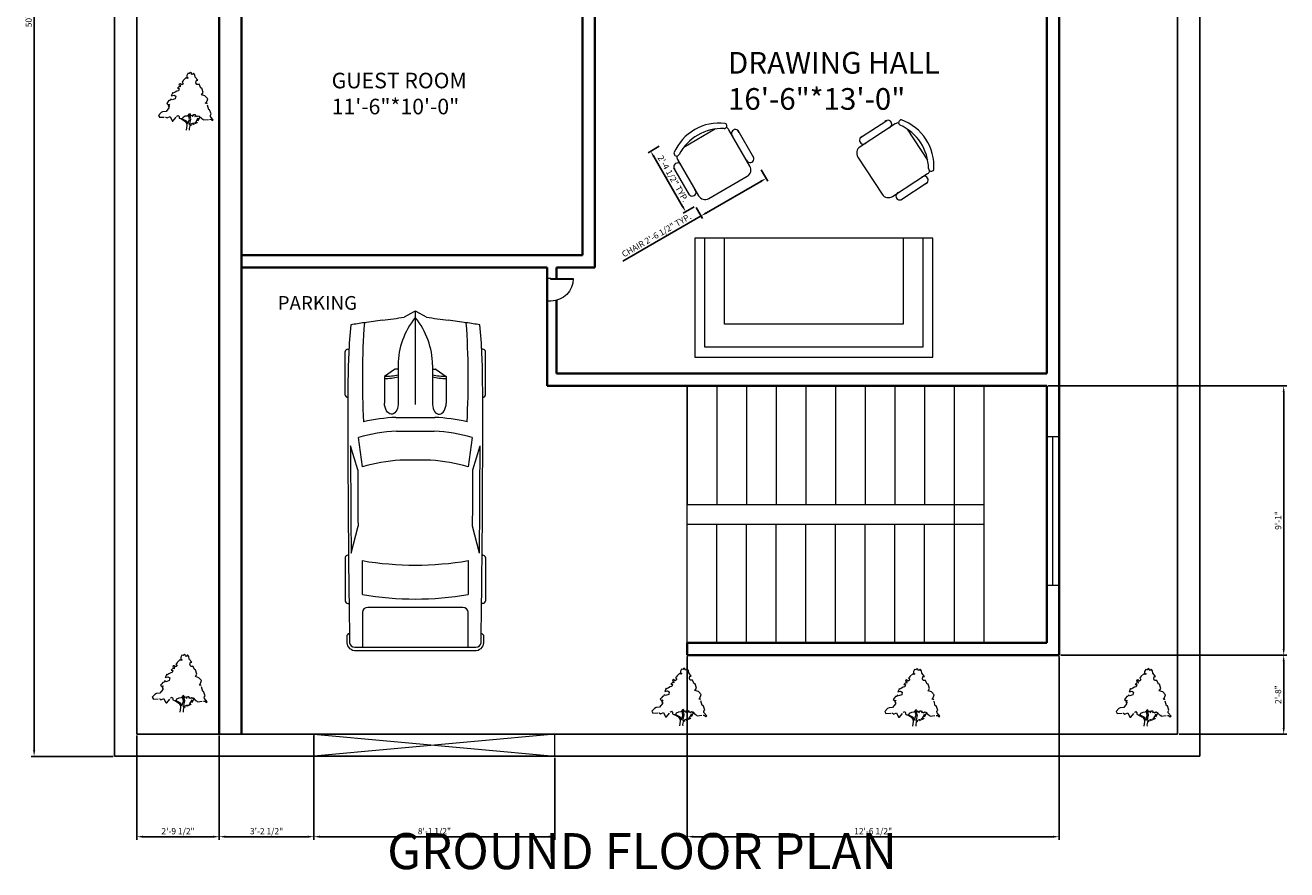
# Model space of a CAD drawing. Units: inches. Extents: x 2432 to 3786, y 1221 to 1905.
# Tile 1 of 4: x 2434 to 2945, y 1221 to 1563. Entities that reach past the tile are written whole.
import ezdxf

# ---------------------------------------------------------------- set-up
doc = ezdxf.new("R2010")
doc.units = ezdxf.units.IN
doc.linetypes.add('ACAD_ISO02W100', pattern=[15, 12, -3])
for name, color, linetype, lineweight, true_color in [('A-ANNO-DIMS', 32, 'Continuous', 18, 0xcd6928), ('A-ANNO-TITL', 40, 'Continuous', 25, 0xf8d731), ('A-AREA-IDEN', 244, 'Continuous', 18, 0x991b1e), ('A-FLOR-STRS', 116, 'Continuous', 18, 0x136734), ('A-FURN', 32, 'Continuous', 13, 0xcd6928), ('A-GLAZ', 116, 'Continuous', 18, 0x136734), ('A-WALL', 67, 'Continuous', 35, 0x727430), ('C-PROP', 67, 'Continuous', 25, 0x727430), ('L-SITE-GATE', 244, 'Continuous', 18, 0x991b1e)]:
    doc.layers.add(name, color=color, linetype=linetype, lineweight=lineweight, true_color=true_color)
for name, color, linetype, lineweight in [('A-DOOR', 4, 'Continuous', 18), ('C-PRKG-VEHC', 8, 'Continuous', 13), ('L-PLNT', 3, 'ACAD_ISO02W100', 13)]:
    doc.layers.add(name, color=color, linetype=linetype, lineweight=lineweight)
doc.styles.get("Standard").update_dxf_attribs({"font": 'arial.ttf'})
doc.dimstyles.new('ISO-25', dxfattribs={"dimtxt": 2.5, "dimasz": 2.5, "dimexe": 1.25, "dimexo": 0.625, "dimtad": 1, "dimdec": 3, "dimlunit": 4, "dimtxsty": 'Standard', "dimcen": 2.5, "dimadec": 0, "dimazin": 0, "dimtfac": 1, "dimtdec": 3, "dimtmove": 0, "dimatfit": 3, "dimfxl": 1, "dimarcsym": 0})

# ---------------------------------------------------------------- blocks, each defined once
blk = doc.blocks.new('*U2')
for p, q in [((21.1, 37.41), (21.1, 36.83)), ((46.55, 38.89), (22.35, 38.89)), ((47.8, 37.39), (47.8, 37.41)), ((87.99, 31.87), (74.76, 35.92)), ((134.31, 35.6), (119.29, 31.78)), ((135.45, 37.07), (135.45, 37.41)), ((136.7, 38.89), (160.9, 38.89)), ((162.15, 37.41), (162.15, 36.77)), ((70.03, 31.54), (86.41, 29.35)), ((138.42, 29.35), (157.25, 29.35)), ((186.47, 29.35), (167.01, 29.35)), ((186.47, -33.5), (186.47, 33.5)), ((188.4, -32.76), (188.4, 32.76)), ((164.52, 26.39), (164.52, -26.39)), ((32.27, 11.63), (36.13, 17.17)), ((36.13, 17.17), (50.94, 17.17)), ((29.77, 9.51), (51.68, 9.51)), ((32.12, 9.51), (32.12, 11.15)), ((58.92, -10.77), (58.92, 10.77)), ((66.55, -10.53), (66.55, 10.53)), ((82.74, 8.5), (82.74, -8.5)), ((186.47, -10.53), (186.47, 10.53)), ((3.27, 6.13), (0.1, 0.41)), ((0, 0), (51.68, 0)), ((0.1, -0.41), (3.27, -6.13)), ((29.77, -9.51), (51.68, -9.51)), ((32.12, -9.51), (32.12, -11.15)), ((32.27, -11.63), (36.13, -17.17)), ((36.13, -17.17), (50.94, -17.17)), ((86.41, -29.35), (70.03, -31.54)), ((87.99, -31.87), (74.76, -35.92)), ((134.31, -35.6), (119.29, -31.78)), ((157.25, -29.35), (138.42, -29.35)), ((167.01, -29.35), (186.47, -29.35)), ((21.1, -37.41), (21.1, -36.83)), ((46.55, -38.89), (22.35, -38.89)), ((47.8, -37.39), (47.8, -37.41)), ((135.45, -37.07), (135.45, -37.41)), ((136.7, -38.89), (160.9, -38.89)), ((162.15, -37.41), (162.15, -36.77))]:
    blk.add_line(p, q)
for centre, major_axis, ratio, start_param, end_param in [((266.03, -27.52), (0, 313.31), 0.842304, 1.367076, 1.39176), ((41.19, -490.86), (0, 528.23), 0.842304, 0.00281, 0.075598), ((22.35, 37.41), (0, -1.48), 0.842304, 3.141593, 4.712389), ((64.48, -10555.62), (0, 10593.03), 0.842304, -0.013397, 0.002797), ((46.55, 37.41), (0, 1.48), 0.842304, -1.570796, 0), ((64.48, -10555.62), (0, -10591.55), 0.842304, 3.133765, 3.140441), ((136.7, 37.41), (0, -1.48), 0.842304, 3.141593, 4.712389), ((160.9, 37.41), (0, 1.48), 0.842304, -1.570796, 0), ((180.63, 35.84), (0, 2.22), 0.842304, -0.013017, 1.249894), ((64.48, -10556.36), (0, 10595.31), 0.842304, -0.013397, -0.013017), ((183.98, 33.5), (0, -2.96), 0.842304, 1.570796, 3.128196), ((183.98, 32.76), (0, -5.25), 0.842304, 1.570796, 3.128196), ((259.18, -27.52), (0, -305.3), 0.842304, 4.528606, 4.561838), ((37.47, -593.96), (0, -623.33), 0.842304, 3.096046, 3.200911), ((134.4, 5.39), (0, -89.78), 0.842304, 4.449482, 4.652344), ((135.29, 5.39), (0, 81.77), 0.842304, 1.245306, 1.50788), ((149.6, 2.8), (0, -79.58), 0.842304, 4.372215, 4.640744), ((95.79, -3666.35), (0, -3698.24), 0.842304, 3.134049, 3.144098), ((17.08, 0), (0, 147.02), 0.842304, 4.511394, 4.913384), ((35.91, 0), (0, 147.02), 0.842304, 4.511394, 4.913384), ((167.01, 26.39), (0, 2.96), 0.842304, 0, 1.570796), ((-204.49, 52.4), (0, -250.96), 0.842304, 1.385369, 1.434372), ((13.04, 17.01), (0, 27.42), 0.842304, 4.435146, 4.718221), ((14.2, 17.01), (0, 27.42), 0.842304, 4.435146, 4.718221), ((50.79, 13.34), (6.34, -0.36), 0.603834, -1.395552, 1.581315), ((29.77, -46.66), (0, 56.17), 0.842304, 0, 0.590319), ((32.75, 11.15), (0, 0.74), 0.842304, 0.879714, 1.570796), ((0.62, 0), (0, -0.74), 0.842304, 4.131459, 5.293319), ((-204.49, -52.4), (0, 250.96), 0.842304, -1.434372, -1.385369), ((29.77, 46.66), (0, 56.17), 0.842304, 2.551274, 3.141593), ((32.75, -11.15), (0, -0.74), 0.842304, 4.712389, 5.403472), ((13.04, -17.01), (0, -27.42), 0.842304, 1.564964, 1.848039), ((14.2, -17.01), (0, -27.42), 0.842304, 1.564964, 1.848039), ((134.4, -5.39), (0, -89.78), 0.842304, -1.510751, -1.307889), ((135.29, -5.39), (0, -81.77), 0.842304, -1.50788, -1.245306), ((149.6, -2.8), (0, -79.58), 0.842304, -1.499151, -1.230623), ((259.18, 27.52), (0, 305.3), 0.842304, 1.721348, 1.754579), ((167.01, -26.39), (0, -2.96), 0.842304, 4.712389, 6.283185), ((266.03, 27.52), (0, 313.31), 0.842304, 1.749832, 1.774517), ((37.47, 593.96), (0, -623.33), 0.842304, -0.059319, 0.045547), ((95.79, 3666.35), (0, -3698.24), 0.842304, -0.002505, 0.007544), ((183.98, -33.5), (0, 2.96), 0.842304, 3.15499, 4.712389), ((183.98, -32.76), (0, -5.25), 0.842304, 0.013397, 1.570796), ((41.19, 490.86), (0, -528.23), 0.842304, -0.075598, -0.00281), ((22.35, -37.41), (0, 1.48), 0.842304, 1.570796, 3.141593), ((64.48, 10555.62), (0, 10593.03), 0.842304, 3.138796, 3.15499), ((46.55, -37.41), (0, -1.48), 0.842304, 0, 1.570796), ((64.48, 10555.62), (0, -10591.55), 0.842304, 0.001152, 0.007828), ((136.7, -37.41), (0, -1.48), 0.842304, -1.570796, 0), ((160.9, -37.41), (0, 1.48), 0.842304, 3.141593, 4.712389), ((180.63, -35.84), (0, -2.22), 0.842304, -1.249894, 0.013017), ((64.48, 10556.36), (0, 10595.31), 0.842304, 3.15461, 3.15499)]:
    blk.add_ellipse(centre, major_axis=major_axis, ratio=ratio, start_param=start_param, end_param=end_param)
at = {"extrusion": (0, 0, -1)}
blk.add_ellipse((50.79, -13.34), major_axis=(6.34, 0.36), ratio=0.603834, start_param=-1.395552, end_param=1.581315, dxfattribs=at)
blk = doc.blocks.new('*U4')
for points in [[(22.0124, 137.721), (18.5475, 141.5624), (15.5282, 138.2446), (13.8028, 139.3505), (13.3714, 142.1153), (11.2148, 143.2214), (8.1954, 140.4564), (4.7447, 141.0094), (2.1567, 136.0326), (2.1567, 131.6088), (5.6074, 129.9499), (3.0193, 128.2909), (0.4313, 130.5029), (-6.9015, 123.3141), (-6.9015, 121.6552), (-9.9208, 119.9963), (-9.0581, 118.3373), (-6.9015, 115.0195), (-10.7835, 112.2546), (-14.6656, 115.0195), (-16.8222, 114.4665), (-17.6849, 112.2546), (-14.6656, 111.7016), (-14.2342, 107.2778), (-17.6065, 107.8307), (-21.5669, 103.9599), (-17.2536, 103.4069), (-18.9789, 97.8771), (-22.8609, 97.3241), (-27.1743, 94.5593), (-32.3504, 91.7944), (-32.7817, 94.0063), (-36.6638, 85.7116), (-29.7624, 87.3705), (-25.449, 84.6056), (-26.743, 77.9699), (-34.507, 75.205), (-37.9578, 77.4169), (-39.2518, 74.099), (-42.2711, 73.5461), (-44.8592, 70.2282), (-47.8786, 66.3574), (-43.9965, 63.0395), (-41.4085, 64.6985), (-44.3346, 59.8898), (-42.2089, 60.1377), (-42.5159, 55.7849), (-49.6039, 46.4502), (-58.2307, 45.8972), (-62.1127, 43.6853), (-68.5828, 36.4966), (-65.9947, 32.0727), (-50.0352, 32.6257), (-47.0159, 30.4138), (-39.6831, 33.7317), (-34.507, 22.6721), (-32.3504, 22.6721), (-22.4296, 34.8376), (-19.4102, 36.4966), (-17.2536, 33.7317), (-17.2536, 29.8608), (-13.8028, 28.7549), (-9.0581, 28.7549), (-7.3328, 32.6257), (-1.7254, 35.3906), (3.8821, 35.9436), (6.4701, 38.1555), (6.9014, 38.7085), (8.1954, 41.4734), (9.9208, 40.3674), (11.2148, 35.9436), (14.2341, 37.6025), (15.0968, 36.4966), (15.9595, 33.7317), (18.9789, 38.7085), (21.9982, 38.7085), (23.2922, 36.4966), (21.9982, 34.2847), (25.4489, 35.3906), (26.743, 33.7317), (29.7623, 35.9436), (32.7817, 34.8376), (38.8204, 28.7549), (41.4084, 27.6489), (43.5651, 25.437), (61.6813, 27.0959), (65.132, 23.7781), (67.7201, 24.884), (60.8186, 33.7317), (60.3873, 37.0495), (62.544, 40.3674), (58.662, 50.874), (56.5053, 50.874), (52.1919, 66.3574), (47.8785, 66.9103), (50.4665, 69.1222), (53.9172, 77.9699), (47.0158, 85.1586), (38.3891, 87.9235), (42.2711, 94.0063)], [(42.2711, 94.0063), (38.8204, 104.5129), (36.6637, 104.5129), (32.3503, 113.9135), (29.7623, 113.3605), (26.743, 113.3605), (24.5862, 117.7844), (25.8802, 123.8671), (29.331, 123.8671), (22.8609, 131.6088), (21.9982, 137.6916)], [(-9.9208, 28.2019), (0, 23.2251), (3.4507, 19.9072), (4.7447, 15.4834), (8.6267, 27.0959), (6.4701, 37.6025)], [(34.5071, 33.1787), (27.1743, 18.2483), (9.0581, 10.5066), (7.7641, 3.8708), (8.1954, 0)], [(8.1954, 40.3674), (11.2148, 27.6489), (8.1954, 13.8245), (24.5862, 19.9072), (32.7817, 34.2847)], [(-12.9401, 28.7549), (-2.588, 22.1191), (0.8626, 17.6953), (1.7253, 11.6125), (0, 0)]]:
    blk.add_lwpolyline(points)
blk = doc.blocks.new('SOFA2')
for p, q in [((-36, 0), (-36, -36)), ((36, 0), (-36, 0)), ((36, -36), (36, 0)), ((-33, -36), (-33, -3)), ((-33, -3), (33, -3)), ((33, -3), (33, -36)), ((-27, -36), (-27, -10)), ((-27, -10), (27, -10)), ((27, -10), (27, -36)), ((-36, -36), (36, -36))]:
    blk.add_line(p, q)
blk = doc.blocks.new('CHAIR7')
for p, q in [((20, 12), (3, 12)), ((5.12, 15.04), (17.88, 15.04)), ((0, 9), (0, -9)), ((23, -7.44), (23, 7.44)), ((3, -12), (20, -12)), ((5.12, -15), (17.88, -15))]:
    blk.add_line(p, q)
for centre, radius, start, end in [((3, 9), 3, 90, 180), ((5.56, 13.54), 1.56, 73.7398, 286.2602), ((17.44, 13.54), 1.56, 253.7398, 106.2602), ((20, 9), 3, 62.4156, 90), ((22.34, 11.12), 1.1, 53.3099, 212.0274), ((4.82, 0), 19.64, 327.5758, 32.4242), ((7, 0), 20, 323.1301, 36.8699), ((3, -9), 3, 180, 270), ((5.56, -13.5), 1.56, 73.7398, 286.2602), ((17.44, -13.5), 1.56, 253.7398, 106.2602), ((20, -9), 3, 270, 297.5844), ((22.34, -11.12), 1.1, 147.9726, 306.6901)]:
    blk.add_arc(centre, radius, start, end)
blk = doc.blocks.new('*U10')
for p, q in [((0, 0), (0, -6)), ((-40, 0), (-40, -6))]:
    blk.add_line(p, q)
blk.add_lwpolyline([(0, 0), (0, 40), (-1.75, 40), (-1.75, 0)], close=True)
blk.add_arc((0, 0), 40, 90, 180)
blk = doc.blocks.new('*D19')
at = {"layer": 'A-ANNO-DIMS', "color": 0, "lineweight": -2, "transparency": 16777216}
for p, q in [((2732.23, 1504.76), (2734.82, 1500.27)), ((2732.03, 1500.1), (2710.02, 1487.39)), ((2705.89, 1489.55), (2708.48, 1485.06)), ((2707.86, 1486.14), (2676.14, 1467.83))]:
    blk.add_line(p, q, dxfattribs=at)
at = {"layer": 'A-ANNO-DIMS', "color": 0, "lineweight": 5, "transparency": 16777216}
for points in [[(2731.82, 1500.46), (2732.24, 1499.74), (2734.2, 1501.35)], [(2709.81, 1487.76), (2710.23, 1487.03), (2707.86, 1486.14)]]:
    blk.add_solid(points, dxfattribs=at)
at = {"layer": 'Defpoints', "color": 0, "lineweight": 5, "transparency": 16777216}
for p in [(2731.92, 1505.3), (2705.58, 1490.1), (2707.86, 1486.14)]:
    blk.add_point(p, dxfattribs=at)
at = {"layer": 'A-ANNO-DIMS', "color": 0, "transparency": 16777216, "insert": (2689.96, 1478.03), "char_height": 2.5, "attachment_point": 5, "rotation": 30}
blk.add_mtext('CHAIR 2\'-6 1/2" TYP.', dxfattribs=at)
blk = doc.blocks.new('*D20')
at = {"layer": 'A-ANNO-DIMS', "color": 0, "lineweight": -2, "transparency": 16777216}
for p, q in [((2690.87, 1514.32), (2686.38, 1511.73)), ((2700.38, 1489.98), (2688.71, 1510.19)), ((2705.04, 1489.78), (2700.54, 1487.19))]:
    blk.add_line(p, q, dxfattribs=at)
at = {"layer": 'A-ANNO-DIMS', "color": 0, "lineweight": 5, "transparency": 16777216}
for points in [[(2689.07, 1510.4), (2688.35, 1509.98), (2687.46, 1512.35)], [(2700.74, 1490.19), (2700.02, 1489.77), (2701.63, 1487.81)]]:
    blk.add_solid(points, dxfattribs=at)
at = {"layer": 'Defpoints', "color": 0, "lineweight": 5, "transparency": 16777216}
for p in [(2687.46, 1512.35), (2691.41, 1514.63), (2705.58, 1490.1)]:
    blk.add_point(p, dxfattribs=at)
at = {"layer": 'A-ANNO-DIMS', "color": 0, "transparency": 16777216, "insert": (2696.2, 1501.04), "char_height": 2.5, "attachment_point": 5, "rotation": 300}
blk.add_mtext('2\'-4 1/2" TYP.', dxfattribs=at)
blk = doc.blocks.new('*D36')
at = {"layer": 'A-ANNO-DIMS', "color": 0, "lineweight": -2, "transparency": 16777216}
for p, q in [((2469.77, 1867.25), (2436.59, 1867.25)), ((2437.84, 1269.75), (2437.84, 1864.75)), ((2469.77, 1267.25), (2436.59, 1267.25))]:
    blk.add_line(p, q, dxfattribs=at)
at = {"layer": 'A-ANNO-DIMS', "color": 0, "lineweight": 5, "transparency": 16777216}
for points in [[(2437.42, 1864.75), (2438.26, 1864.75), (2437.84, 1867.25)], [(2437.42, 1269.75), (2438.26, 1269.75), (2437.84, 1267.25)]]:
    blk.add_solid(points, dxfattribs=at)
at = {"layer": 'Defpoints', "color": 0, "lineweight": 5, "transparency": 16777216}
for p in [(2437.84, 1867.25), (2470.39, 1867.25), (2470.39, 1267.25)]:
    blk.add_point(p, dxfattribs=at)
at = {"layer": 'A-ANNO-DIMS', "color": 0, "transparency": 16777216, "insert": (2435.94, 1567.25), "char_height": 2.5, "attachment_point": 5, "rotation": 90}
blk.add_mtext('50\'-0"', dxfattribs=at)
blk = doc.blocks.new('*D37')
at = {"layer": 'A-ANNO-DIMS', "color": 0, "lineweight": -2, "transparency": 16777216}
for p, q in [((2479.39, 1275.63), (2479.39, 1233.45)), ((2512.8, 1275.63), (2512.8, 1233.45)), ((2481.89, 1234.7), (2510.3, 1234.7))]:
    blk.add_line(p, q, dxfattribs=at)
at = {"layer": 'A-ANNO-DIMS', "color": 0, "lineweight": 5, "transparency": 16777216}
for points in [[(2481.89, 1235.12), (2481.89, 1234.28), (2479.39, 1234.7)], [(2510.3, 1235.12), (2510.3, 1234.28), (2512.8, 1234.7)]]:
    blk.add_solid(points, dxfattribs=at)
at = {"layer": 'Defpoints', "color": 0, "lineweight": 5, "transparency": 16777216}
for p in [(2479.39, 1276.25), (2512.8, 1276.25), (2512.8, 1234.7)]:
    blk.add_point(p, dxfattribs=at)
at = {"layer": 'A-ANNO-DIMS', "color": 0, "transparency": 16777216, "insert": (2496.09, 1236.62), "char_height": 2.5, "attachment_point": 5}
blk.add_mtext('2\'-9 1/2"', dxfattribs=at)
blk = doc.blocks.new('*D38')
at = {"layer": 'A-ANNO-DIMS', "color": 0, "lineweight": -2, "transparency": 16777216}
for p, q in [((2848.42, 1417.25), (2944.97, 1417.25)), ((2943.72, 1310.75), (2943.72, 1414.75)), ((2853.45, 1308.25), (2944.97, 1308.25))]:
    blk.add_line(p, q, dxfattribs=at)
at = {"layer": 'A-ANNO-DIMS', "color": 0, "lineweight": 5, "transparency": 16777216}
for points in [[(2943.31, 1414.75), (2944.14, 1414.75), (2943.72, 1417.25)], [(2943.31, 1310.75), (2944.14, 1310.75), (2943.72, 1308.25)]]:
    blk.add_solid(points, dxfattribs=at)
at = {"layer": 'Defpoints', "color": 0, "lineweight": 5, "transparency": 16777216}
for p in [(2847.8, 1417.25), (2943.72, 1417.25), (2852.82, 1308.25)]:
    blk.add_point(p, dxfattribs=at)
at = {"layer": 'A-ANNO-DIMS', "color": 0, "transparency": 16777216, "insert": (2941.82, 1362.75), "char_height": 2.5, "attachment_point": 5, "rotation": 90}
blk.add_mtext('9\'-1"', dxfattribs=at)
blk = doc.blocks.new('*D39')
at = {"layer": 'A-ANNO-DIMS', "color": 0, "lineweight": -2, "transparency": 16777216}
for p, q in [((2853.45, 1308.25), (2944.97, 1308.25)), ((2943.72, 1305.75), (2943.72, 1278.75)), ((2901.42, 1276.25), (2944.97, 1276.25))]:
    blk.add_line(p, q, dxfattribs=at)
at = {"layer": 'A-ANNO-DIMS', "color": 0, "lineweight": 5, "transparency": 16777216}
for points in [[(2943.31, 1305.75), (2944.14, 1305.75), (2943.72, 1308.25)], [(2943.31, 1278.75), (2944.14, 1278.75), (2943.72, 1276.25)]]:
    blk.add_solid(points, dxfattribs=at)
at = {"layer": 'Defpoints', "color": 0, "lineweight": 5, "transparency": 16777216}
for p in [(2852.82, 1308.25), (2900.8, 1276.25), (2943.72, 1276.25)]:
    blk.add_point(p, dxfattribs=at)
at = {"layer": 'A-ANNO-DIMS', "color": 0, "transparency": 16777216, "insert": (2941.82, 1292.25), "char_height": 2.5, "attachment_point": 5, "rotation": 90}
blk.add_mtext('2\'-8"', dxfattribs=at)
blk = doc.blocks.new('*D40')
at = {"layer": 'A-ANNO-DIMS', "color": 0, "lineweight": -2, "transparency": 16777216}
for p, q in [((2702.21, 1307.62), (2702.21, 1233.45)), ((2852.82, 1307.63), (2852.82, 1233.45)), ((2704.71, 1234.7), (2850.32, 1234.7))]:
    blk.add_line(p, q, dxfattribs=at)
at = {"layer": 'A-ANNO-DIMS', "color": 0, "lineweight": 5, "transparency": 16777216}
for points in [[(2704.71, 1235.12), (2704.71, 1234.28), (2702.21, 1234.7)], [(2850.32, 1235.12), (2850.32, 1234.28), (2852.82, 1234.7)]]:
    blk.add_solid(points, dxfattribs=at)
at = {"layer": 'Defpoints', "color": 0, "lineweight": 5, "transparency": 16777216}
for p in [(2702.21, 1308.25), (2852.82, 1308.25), (2852.82, 1234.7)]:
    blk.add_point(p, dxfattribs=at)
at = {"layer": 'A-ANNO-DIMS', "color": 0, "transparency": 16777216, "insert": (2777.52, 1236.62), "char_height": 2.5, "attachment_point": 5}
blk.add_mtext('12\'-6 1/2"', dxfattribs=at)
blk = doc.blocks.new('*D41')
at = {"layer": 'A-ANNO-DIMS', "color": 0, "lineweight": -2, "transparency": 16777216}
for p, q in [((2551.09, 1266.63), (2551.09, 1233.45)), ((2648.7, 1266.63), (2648.7, 1233.45)), ((2553.59, 1234.7), (2646.2, 1234.7))]:
    blk.add_line(p, q, dxfattribs=at)
at = {"layer": 'A-ANNO-DIMS', "color": 0, "lineweight": 5, "transparency": 16777216}
for points in [[(2553.59, 1235.12), (2553.59, 1234.28), (2551.09, 1234.7)], [(2646.2, 1235.12), (2646.2, 1234.28), (2648.7, 1234.7)]]:
    blk.add_solid(points, dxfattribs=at)
at = {"layer": 'Defpoints', "color": 0, "lineweight": 5, "transparency": 16777216}
for p in [(2551.09, 1267.25), (2648.7, 1267.25), (2648.7, 1234.7)]:
    blk.add_point(p, dxfattribs=at)
at = {"layer": 'A-ANNO-DIMS', "color": 0, "transparency": 16777216, "insert": (2599.9, 1236.62), "char_height": 2.5, "attachment_point": 5}
blk.add_mtext('8\'-1 1/2"', dxfattribs=at)
blk = doc.blocks.new('*D42')
at = {"layer": 'A-ANNO-DIMS', "color": 0, "lineweight": -2, "transparency": 16777216}
for p, q in [((2512.8, 1275.63), (2512.8, 1233.45)), ((2551.09, 1275.63), (2551.09, 1233.45)), ((2515.3, 1234.7), (2548.59, 1234.7))]:
    blk.add_line(p, q, dxfattribs=at)
at = {"layer": 'A-ANNO-DIMS', "color": 0, "lineweight": 5, "transparency": 16777216}
for points in [[(2515.3, 1235.12), (2515.3, 1234.28), (2512.8, 1234.7)], [(2548.59, 1235.12), (2548.59, 1234.28), (2551.09, 1234.7)]]:
    blk.add_solid(points, dxfattribs=at)
at = {"layer": 'Defpoints', "color": 0, "lineweight": 5, "transparency": 16777216}
for p in [(2512.8, 1276.25), (2551.09, 1276.25), (2551.09, 1234.7)]:
    blk.add_point(p, dxfattribs=at)
at = {"layer": 'A-ANNO-DIMS', "color": 0, "transparency": 16777216, "insert": (2531.94, 1236.62), "char_height": 2.5, "attachment_point": 5}
blk.add_mtext('3\'-2 1/2"', dxfattribs=at)

msp = doc.modelspace()

# ---------------------------------------------------------------- linework, layer by layer
at = {"layer": 'A-FLOR-STRS'}
for p, q in [((2702.2654, 1313.2516), (2702.2654, 1417.2516)), ((2702.2654, 1417.2516), (2702.2654, 1369.2516)), ((2714.2654, 1417.2516), (2714.2654, 1369.2516)), ((2726.2654, 1417.2516), (2726.2654, 1369.2516)), ((2738.2654, 1417.2516), (2738.2654, 1369.2516)), ((2750.2654, 1417.2516), (2750.2654, 1369.2516)), ((2762.2654, 1417.2516), (2762.2654, 1369.2516)), ((2774.2654, 1417.2516), (2774.2654, 1369.2516)), ((2786.2654, 1417.2516), (2786.2654, 1369.2516)), ((2798.2654, 1417.2516), (2798.2654, 1369.2516)), ((2810.2654, 1417.2516), (2810.2654, 1369.2516)), ((2822.2654, 1417.2516), (2822.2654, 1369.2516)), ((2702.2654, 1369.2516), (2822.2654, 1369.2516)), ((2810.2654, 1369.2516), (2810.2654, 1313.2516)), ((2822.2654, 1369.2516), (2822.2654, 1313.2516)), ((2702.2654, 1313.2516), (2702.2654, 1361.2516)), ((2702.2654, 1361.2516), (2822.2654, 1361.2516)), ((2714.2654, 1313.2516), (2714.2654, 1361.2516)), ((2726.2654, 1313.2516), (2726.2654, 1361.2516)), ((2738.2654, 1313.2516), (2738.2654, 1361.2516)), ((2750.2654, 1313.2516), (2750.2654, 1361.2516)), ((2762.2654, 1313.2516), (2762.2654, 1361.2516)), ((2774.2654, 1313.2516), (2774.2654, 1361.2516)), ((2786.2654, 1313.2516), (2786.2654, 1361.2516)), ((2798.2654, 1313.2516), (2798.2654, 1361.2516)), ((2847.7964, 1313.2516), (2702.2654, 1313.2516)), ((2852.824, 1313.2516), (2852.7964, 1313.2516))]:
    msp.add_line(p, q, dxfattribs=at)
at = {"layer": 'A-GLAZ'}
for p, q in [((2847.7964, 1336.4718), (2847.7964, 1396.811)), ((2847.7964, 1396.811), (2852.7964, 1396.811)), ((2850.2964, 1336.4718), (2850.2964, 1396.811)), ((2852.7964, 1396.811), (2852.7964, 1336.4718)), ((2852.7964, 1336.4718), (2847.7964, 1336.4718)), ((2852.7964, 1336.4718), (2850.2964, 1336.4718))]:
    msp.add_line(p, q, dxfattribs=at)
at = {"layer": 'A-WALL'}
for p, q in [((2512.7964, 1276.2516), (2512.7964, 1715.2516)), ((2521.7964, 1276.2516), (2521.7964, 1715.2516)), ((2852.7964, 1715.2516), (2852.7964, 1422.2516)), ((2664.7964, 1590.2516), (2664.7964, 1470.2516)), ((2847.7964, 1422.2516), (2847.7964, 1578.2516)), ((2659.7964, 1572.3142), (2659.7964, 1470.2516)), ((2659.7964, 1470.2516), (2521.7964, 1470.2516)), ((2664.7964, 1465.2516), (2664.7964, 1470.2516)), ((2645.6067, 1465.2516), (2521.7964, 1465.2516)), ((2645.6067, 1417.2516), (2645.6067, 1465.2516)), ((2659.7964, 1465.2516), (2649.2822, 1465.2516)), ((2649.2822, 1460.7758), (2649.2822, 1465.2516)), ((2659.7964, 1465.2516), (2664.7964, 1465.2516)), ((2649.2822, 1422.2516), (2649.2822, 1451.9546)), ((2652.8527, 1422.2516), (2649.2822, 1422.2516)), ((2708.7964, 1422.2516), (2652.8527, 1422.2516)), ((2708.7964, 1422.2516), (2847.7964, 1422.2516)), ((2852.7964, 1417.2516), (2852.7964, 1422.2516)), ((2708.7964, 1417.2516), (2645.6067, 1417.2516)), ((2708.7964, 1417.2516), (2822.2654, 1417.2516)), ((2822.2654, 1417.2516), (2847.7964, 1417.2516)), ((2847.7964, 1417.2516), (2847.7964, 1313.2516)), ((2852.7964, 1417.2516), (2852.7964, 1313.2516)), ((2847.7964, 1313.2516), (2702.2654, 1313.2516)), ((2702.2654, 1313.2516), (2702.2654, 1308.2516)), ((2852.824, 1308.2516), (2852.824, 1313.2516)), ((2702.2654, 1308.2516), (2852.824, 1308.2516))]:
    msp.add_line(p, q, dxfattribs=at)
at = {"layer": 'C-PROP'}
for p, q in [((2470.3906, 1267.2516), (2470.3906, 1867.2516)), ((2909.7964, 1267.2516), (2909.7964, 1867.2516)), ((2479.3906, 1276.2516), (2479.3906, 1858.2516)), ((2900.7964, 1276.2516), (2900.7964, 1769.2516)), ((2900.7964, 1276.2516), (2479.3906, 1276.2516)), ((2909.7964, 1267.2516), (2470.3906, 1267.2516))]:
    msp.add_line(p, q, dxfattribs=at)
at = {"layer": 'L-SITE-GATE'}
for p, q in [((2551.0932, 1276.2516), (2551.0932, 1267.2516)), ((2648.6987, 1276.2516), (2551.0932, 1276.2516)), ((2551.0932, 1276.2516), (2648.6987, 1267.2516)), ((2648.6987, 1276.2516), (2551.0932, 1267.2516)), ((2648.6987, 1267.2516), (2648.6987, 1276.2516)), ((2648.6987, 1267.2516), (2648.6987, 1276.2516)), ((2551.0932, 1267.2516), (2648.6987, 1267.2516))]:
    msp.add_line(p, q, dxfattribs=at)

# ---------------------------------------------------------------- block references
at = {"layer": 'A-DOOR', "xscale": -0.2277050421196423, "yscale": 0.2277050421196423, "zscale": 0.2277050421196423, "rotation": 270}
msp.add_blockref('*U10', (2647.0134, 1460.7758), dxfattribs=at)
at = {"layer": 'A-FURN'}
for p, rotation in [((2718.7649, 1497.7099), 119.999999999999), ((2776.2642, 1502.4341), 33.07624776584069)]:
    msp.add_blockref('CHAIR7', p, dxfattribs=dict(at, rotation=rotation))
at = {"layer": 'A-FURN', "xscale": 1.338107814876162, "yscale": 1.338107814876162, "zscale": 1.338107814876162, "rotation": 180.0000000000001}
msp.add_blockref('SOFA2', (2753.5136, 1428.8995), dxfattribs=at)
at = {"layer": 'C-PRKG-VEHC', "xscale": 0.7296570802088281, "yscale": 0.7296570802088281, "zscale": 0.7296570802088281, "rotation": 270}
msp.add_blockref('*U2', (2592.162, 1447.5237), dxfattribs=at)
at = {"layer": 'L-PLNT', "xscale": 0.163121370253731, "yscale": 0.163121370253731, "zscale": 0.163121370253731}
for p in [(2499.3346, 1520.854), (2496.8675, 1285.2019), (2699.1101, 1279.5552), (2793.4653, 1279.4317), (2887.0799, 1279.4317)]:
    msp.add_blockref('*U4', p, dxfattribs=at)

# ---------------------------------------------------------------- texts
at = {"layer": 'A-ANNO-TITL', "insert": (2580.7849, 1236.15), "char_height": 14.590252, "attachment_point": 1}
msp.add_mtext_dynamic_manual_height_columns('GROUND FLOOR PLAN', width=282.090868, gutter_width=72.9513, heights=[0], dxfattribs=at)
at = {"layer": 'A-AREA-IDEN', "attachment_point": 1}
for s, width, gutter_width, insert, char_height in [('DRAWING HALL\\P16\'-6"*13\'-0"', 275.489243, 43.9033, (2718.7239, 1552.5418), 8.780661), ('GUEST ROOM\\P11\'-6"*10\'-0"', 147.164718, 31.5753, (2558.2909, 1544.1293), 6.315062), ('PARKING', 72.047362, 27.8562, (2536.4324, 1453.6833), 5.57124)]:
    msp.add_mtext_dynamic_manual_height_columns(s, width=width, gutter_width=gutter_width, heights=[0], dxfattribs=dict(at, insert=insert, char_height=char_height))

# ---------------------------------------------------------------- dimensions: what is measured, and where the dimension line sits
at = {"layer": 'A-ANNO-DIMS'}
for base, p1, p2, picture, middle in [((2437.8406, 1867.2516), (2470.3906, 1267.2516), (2470.3906, 1867.2516), '*D36', (2435.9391, 1567.2516)), ((2943.7221, 1417.2516), (2852.824, 1308.2516), (2847.7964, 1417.2516), '*D38', (2941.8207, 1362.7516)), ((2943.7221, 1276.2516), (2852.824, 1308.2516), (2900.7964, 1276.2516), '*D39', (2941.8207, 1292.2516))]:
    dim = msp.add_linear_dim(base=base, p1=p1, p2=p2, angle=90, dimstyle='ISO-25', override={"dimdec": 1, "dimlfac": 1, "dimrnd": 0, "dimzin": 1, "dimdsep": 46, "dimlunit": 4, "dimfrac": 2}, dxfattribs=at)
    dim.commit()
    dim.dimension.update_dxf_attribs({"geometry": picture, "text_midpoint": middle})
for base, p1, p2, angle, text, picture, middle in [((2687.4592, 1512.3521), (2705.5768, 1490.0958), (2691.4102, 1514.6332), 120, '<> TYP.', '*D20', (2696.2032, 1501.0422)), ((2707.8579, 1486.1448), (2731.9166, 1505.3031), (2705.5768, 1490.0958), 210, 'CHAIR <> TYP.', '*D19', (2689.9589, 1478.0251))]:
    dim = msp.add_linear_dim(base=base, p1=p1, p2=p2, angle=angle, text=text, dimstyle='ISO-25', override={"dimdec": 1, "dimlfac": 1, "dimrnd": 0, "dimzin": 1, "dimdsep": 46, "dimlunit": 4, "dimfrac": 2}, dxfattribs=at)
    dim.commit()
    dim.dimension.update_dxf_attribs({"geometry": picture, "text_midpoint": middle})
for base, p1, p2, picture, middle in [((2852.824, 1234.7016), (2702.2064, 1308.2468), (2852.824, 1308.2516), '*D40', (2777.5152, 1236.6192)), ((2512.7964, 1234.7016), (2479.3906, 1276.2516), (2512.7964, 1276.2516), '*D37', (2496.0935, 1236.6192)), ((2551.0932, 1234.7016), (2512.7964, 1276.2516), (2551.0932, 1276.2516), '*D42', (2531.9448, 1236.6201)), ((2648.6987, 1234.7016), (2551.0932, 1267.2516), (2648.6987, 1267.2516), '*D41', (2599.896, 1236.6192))]:
    dim = msp.add_linear_dim(base=base, p1=p1, p2=p2, dimstyle='ISO-25', override={"dimdec": 1, "dimlfac": 1, "dimrnd": 0, "dimzin": 1, "dimdsep": 46, "dimlunit": 4, "dimfrac": 2}, dxfattribs=at)
    dim.commit()
    dim.dimension.update_dxf_attribs({"geometry": picture, "text_midpoint": middle})

doc.saveas('drawing.dxf')
